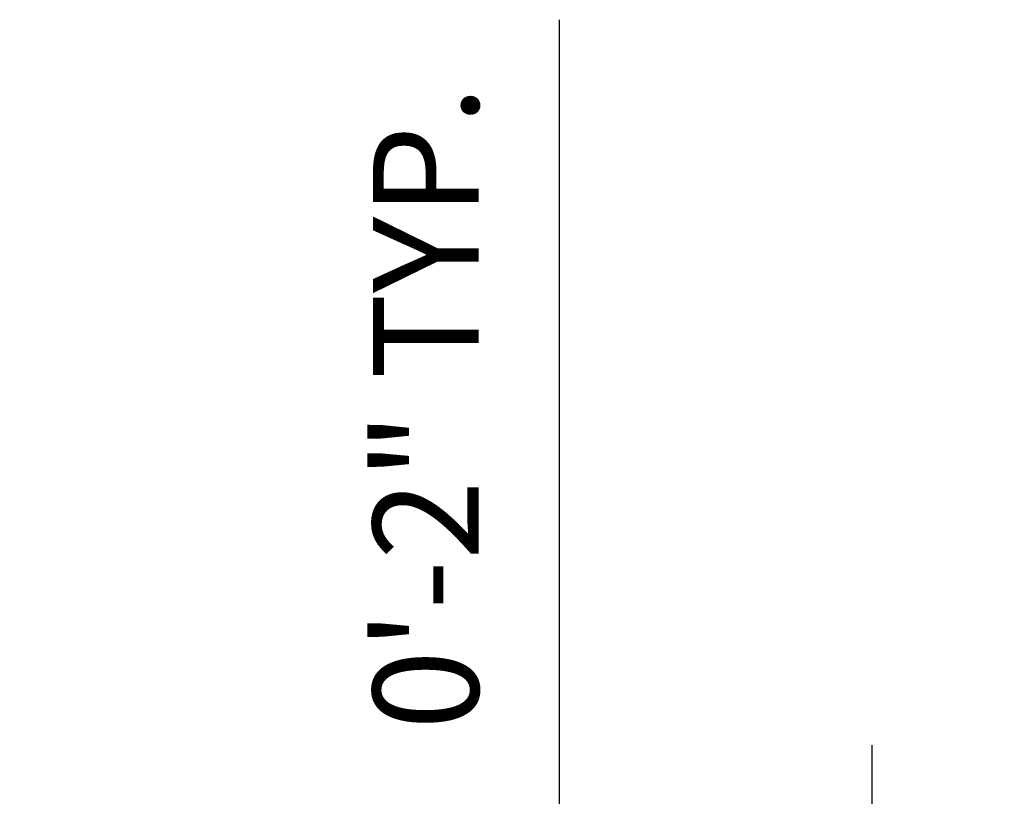
# Model space of a CAD drawing. Units: millimetres. Extents: x 7894 to 8038, y 6851 to 6951.
# Tile 15 of 49: x 7974.616 to 7983.933, y 6885.337 to 6892.689. Entities that reach past the tile are written whole.
import ezdxf

# ---------------------------------------------------------------- set-up
doc = ezdxf.new("R2010")
doc.units = ezdxf.units.MM
doc.layers.add('A-ANNO-DIMS', color=2, linetype='Continuous', lineweight=18)
doc.styles.get("Standard").update_dxf_attribs({"font": 'arial.ttf'})
doc.dimstyles.new('ISO-25', dxfattribs={"dimtxt": 1, "dimasz": 1, "dimexe": 1.25, "dimexo": 0.625, "dimtad": 1, "dimdec": 0, "dimlunit": 4, "dimtxsty": 'Standard', "dimcen": 2.5, "dimclrt": 1, "dimadec": 0, "dimazin": 0, "dimtfac": 1, "dimtdec": 0, "dimtmove": 0, "dimatfit": 3, "dimfxl": 1, "dimarcsym": 0})

# ---------------------------------------------------------------- blocks, each defined once
blk = doc.blocks.new('*D20')
at = {"layer": 'A-ANNO-DIMS', "color": 0, "lineweight": -2, "transparency": 16777216}
for p, q in [((7979.7235, 6884.3436), (7979.7235, 6892.6891)), ((7979.7235, 6881.3545), (7979.7235, 6883.3436)), ((7979.9825, 6883.3436), (7980.9735, 6883.3436)), ((7979.9825, 6881.3545), (7980.9735, 6881.3545)), ((7979.7235, 6880.3545), (7979.7235, 6879.3545))]:
    blk.add_line(p, q, dxfattribs=at)
at = {"layer": 'A-ANNO-DIMS', "color": 0, "transparency": 16777216}
for points in [[(7979.5568, 6884.3436), (7979.8902, 6884.3436), (7979.7235, 6883.3436)], [(7979.5568, 6880.3545), (7979.8902, 6880.3545), (7979.7235, 6881.3545)]]:
    blk.add_solid(points, dxfattribs=at)
at = {"layer": 'Defpoints', "color": 0, "transparency": 16777216}
for p in [(7979.3575, 6883.3436), (7979.7235, 6883.3436), (7979.3575, 6881.3545)]:
    blk.add_point(p, dxfattribs=at)
at = {"layer": 'A-ANNO-DIMS', "color": 1, "transparency": 16777216, "insert": (7978.5879, 6889.0163), "char_height": 1, "attachment_point": 5, "rotation": 90}
blk.add_mtext('0\'-2" TYP.', dxfattribs=at)
blk = doc.blocks.new('*D40')
at = {"layer": 'A-ANNO-DIMS', "color": 0, "lineweight": -2, "transparency": 16777216}
for p, q in [((7982.6834, 6878.5836), (7982.6834, 6885.822)), ((7981.4609, 6878.5836), (7983.9334, 6878.5836)), ((7982.6834, 6874.8578), (7982.6834, 6877.5836)), ((7964.1574, 6873.8578), (7983.9334, 6873.8578))]:
    blk.add_line(p, q, dxfattribs=at)
at = {"layer": 'A-ANNO-DIMS', "color": 0, "transparency": 16777216}
for points in [[(7982.5168, 6877.5836), (7982.8501, 6877.5836), (7982.6834, 6878.5836)], [(7982.5168, 6874.8578), (7982.8501, 6874.8578), (7982.6834, 6873.8578)]]:
    blk.add_solid(points, dxfattribs=at)
at = {"layer": 'Defpoints', "color": 0, "transparency": 16777216}
for p in [(7980.8359, 6878.5836), (7982.6834, 6878.5836), (7963.5324, 6873.8578)]:
    blk.add_point(p, dxfattribs=at)
at = {"layer": 'A-ANNO-DIMS', "color": 1, "transparency": 16777216, "insert": (7981.5414, 6882.7028), "char_height": 1, "attachment_point": 5, "rotation": 90}
blk.add_mtext('0\'-4 1/2"', dxfattribs=at)

msp = doc.modelspace()

# ---------------------------------------------------------------- dimensions: what is measured, and where the dimension line sits
at = {"layer": 'A-ANNO-DIMS'}
dim = msp.add_linear_dim(base=(7979.7235, 6883.3436), p1=(7979.3575, 6881.3545), p2=(7979.3575, 6883.3436), angle=90, text='<> TYP.', dimstyle='ISO-25', override={"dimdec": 1, "dimlfac": 1, "dimrnd": 0, "dimzin": 1, "dimdsep": 46, "dimlunit": 4, "dimfrac": 2}, dxfattribs=at)
dim.commit()
dim.dimension.update_dxf_attribs({"geometry": '*D20', "text_midpoint": (7978.5879, 6889.0163)})
dim = msp.add_linear_dim(base=(7982.6834, 6878.5836), p1=(7963.5324, 6873.8578), p2=(7980.8359, 6878.5836), angle=90, dimstyle='ISO-25', override={"dimdec": 1, "dimlfac": 1, "dimrnd": 0, "dimzin": 1, "dimdsep": 46, "dimlunit": 4, "dimfrac": 2}, dxfattribs=at)
dim.commit()
dim.dimension.update_dxf_attribs({"geometry": '*D40', "text_midpoint": (7981.5414, 6882.7028)})

doc.saveas('drawing.dxf')
